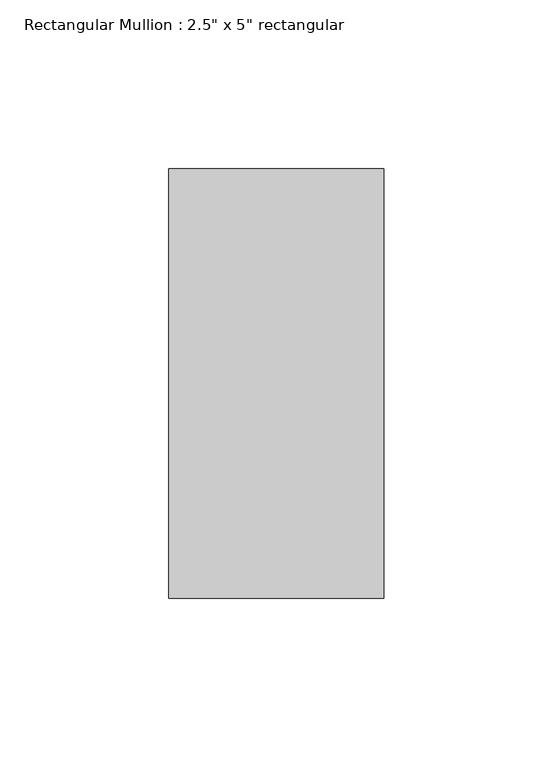
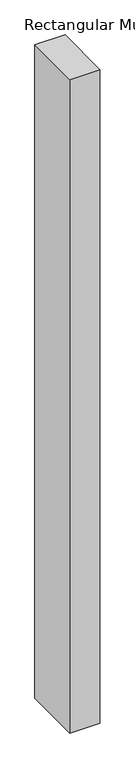
"""IFC4 building model written with IfcOpenShell, lengths in millimetres: member geometry."""

from ifc_helpers import new_model, si_unit, frame, origin, place, context, project, spatial, polyline, outline, extrude, source, transform, mapped, element, save


def member_0700671e(model_context):
    return source(origin(), model_context, "Body", "SweptSolid", [
        extrude(outline(polyline([(31.75, 63.5), (31.75, -63.5), (-31.75, -63.5), (-31.75, 63.5), (31.75, 63.5)])), frame((0.0, 0.0, -1454.3964565), z_axis=(0.0, 0.0, 1.0), x_axis=(1.0, 0.0, 0.0)), (0.0, 0.0, 1.0), 1454.3964565),
    ])


if __name__ == "__main__":
    model = new_model("IFC4")
    model_context = context("Model", 3, world=origin())
    ifc_project = project(units=[si_unit("LENGTHUNIT", "METRE", prefix="MILLI")], contexts=[model_context])
    site = spatial("IfcSite", under=ifc_project)
    building = spatial("IfcBuilding", under=site)
    placement = place(None, origin())
    member_shape = member_0700671e(model_context)
    element("IfcMember", 1, ObjectType="Rectangular Mullion : 2.5\" x 5\" rectangular", at=placement, inside=building, context=model_context, shape_type="MappedRepresentation", body=[
        mapped(member_shape, transform((0.0, 0.0, 0.0), x_axis=(1.0, 0.0, 0.0), y_axis=(0.0, 1.0, 0.0), z_axis=(0.0, 0.0, 1.0))),
    ])
    save(model, "model.ifc")

# Revit data of these elements
# Type "Rectangular Mullion : 2.5\" x 5\" rectangular"
#   built-in parameter 1007304 = 0.416667 (stored number, unit not read)
#   built-in parameter 1007301 = 0.104167 (stored number, unit not read)
#   built-in parameter 1007300 = 0.104167 (stored number, unit not read)
# Element 1 (IfcMember, "Rectangular Mullion : 2.5\" x 5\" rectangular")
#   Materials on its faces: "Aluminum"
# Materials
#   "Aluminum": class "Metal", colour RGB 247 247 247, transparency 0, Description = "Aluminum 6061", Cost = 0
